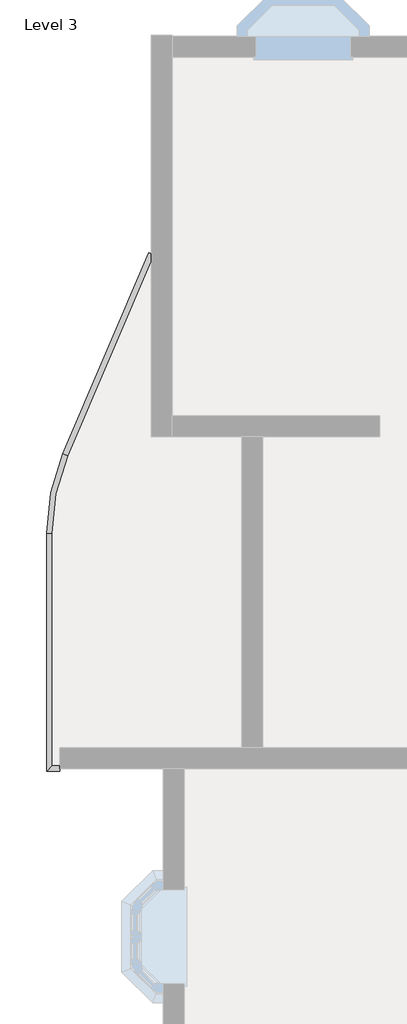
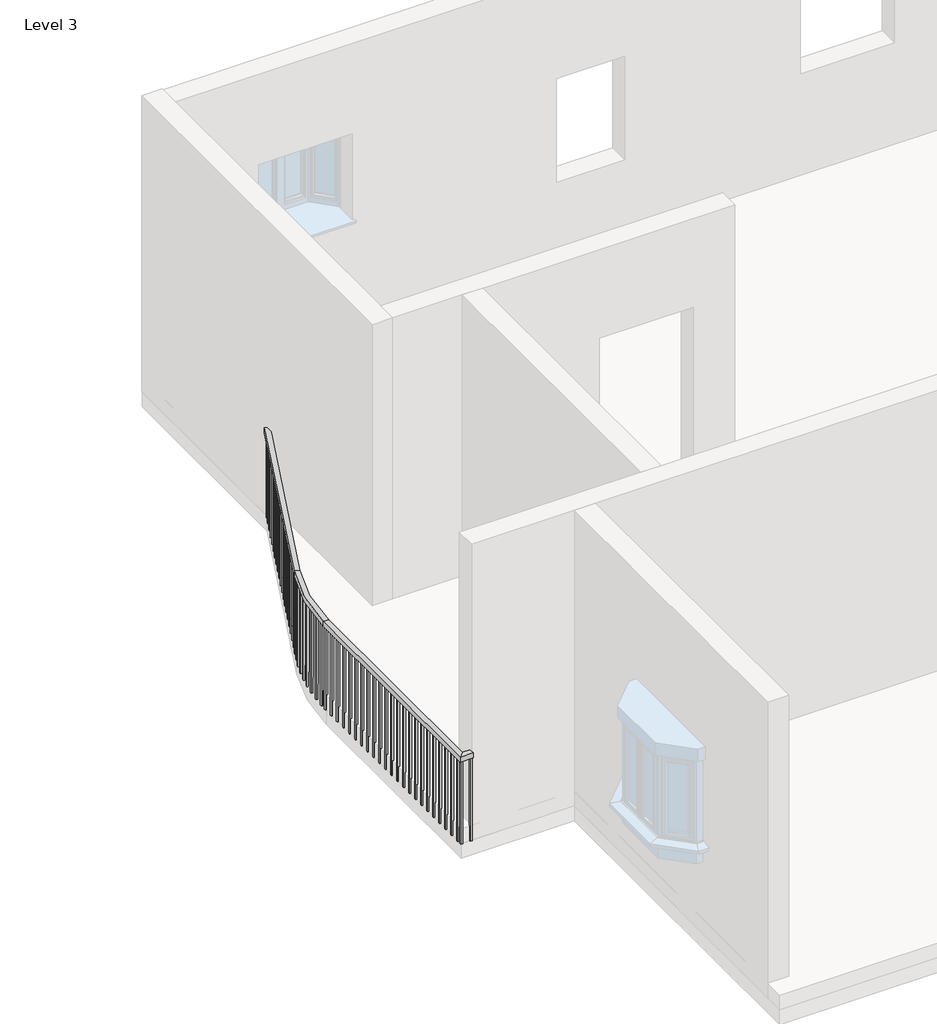
# One storey, part 7 of 14: 1 railing.
"""IFC4 building model written with IfcOpenShell, lengths in millimetres."""

from ifc_helpers import new_model, si_unit, frame, origin, place, context, project, spatial, polyline, circle_curve, outline, extrude, element, save
from ifc_brep_helpers import plane_surface, cylinder_surface, revolved_surface, advanced_brep

model = new_model("IFC4")

# Units and contexts
model_context = context("Model", 3, world=origin())
ifc_project = project(units=[si_unit("LENGTHUNIT", "METRE", prefix="MILLI")], contexts=[model_context])

# Site, building, storey
site = spatial("IfcSite", under=ifc_project)
building = spatial("IfcBuilding", under=site)
storey = spatial("IfcBuildingStorey", under=building, Name="Level 3", Elevation=6096.0)

# Railing
placement = place(None, origin())
element("IfcRailing", 1, ObjectType="Handrail - Rectangular", at=placement, inside=storey, context=model_context, shape_type="SolidModel", body=[
    advanced_brep(
    [(-12381.4379579, -2441.2590879, 7010.4), (-12381.4379579, -2441.2590879, 6959.6), (-12428.1364721, -2421.2618688, 6959.6), (-12428.1364721, -2421.2618688, 7010.4), (-13216.1814979, -4390.5942894, 7010.4), (-13216.1814979, -4390.5942894, 6959.6), (-13262.8800121, -4370.5970703, 6959.6), (-13262.8800121, -4370.5970703, 7010.4), (-13369.987215, -5140.4900045, 6959.6), (-13369.987215, -5140.4900045, 7010.4), (-13420.787215, -5140.4900045, 6959.6), (-13420.787215, -5140.4900045, 7010.4), (-13369.987215, -7396.5416506, 7010.4), (-13369.987215, -7396.5416506, 6959.6), (-13420.787215, -7447.3416506, 6959.6), (-13420.787215, -7447.3416506, 7010.4), (-13293.787215, -7396.5416506, 7010.4), (-13293.787215, -7447.3416506, 7010.4), (-13293.787215, -7447.3416506, 6959.6), (-13293.787215, -7396.5416506, 6959.6)],
    [
        (0, 1),
        (1, 2),
        (2, 3),
        (3, 0),
        (0, 4),
        (4, 5),
        (5, 1),
        (5, 6),
        (6, 2),
        (6, 7),
        (7, 3),
        (7, 4),
        (8, 5, circle_curve(frame((-11464.987215, -5140.4900045, 6959.6), z_axis=(0.0, 0.0, -1.0), x_axis=(-0.9192620907623801, 0.39364604467361003, 0.0)), 1905.0)),
        (4, 9, circle_curve(frame((-11464.987215, -5140.4900045, 7010.4), z_axis=(0.0, 0.0, 1.0), x_axis=(-0.9192620907623801, 0.39364604467361003, 0.0)), 1905.0)),
        (9, 8),
        (10, 6, circle_curve(frame((-11464.987215, -5140.4900045, 6959.6), z_axis=(0.0, 0.0, -1.0), x_axis=(-0.9192620907623801, 0.39364604467361003, 0.0)), 1955.8)),
        (8, 10),
        (11, 7, circle_curve(frame((-11464.987215, -5140.4900045, 7010.4), z_axis=(0.0, 0.0, -1.0), x_axis=(-0.9192620907623801, 0.39364604467361003, 0.0)), 1955.8)),
        (10, 11),
        (11, 9),
        (9, 12),
        (12, 13),
        (13, 8),
        (13, 14),
        (14, 10),
        (14, 15),
        (15, 11),
        (15, 12),
        (16, 17),
        (17, 18),
        (18, 19),
        (19, 16),
        (12, 16),
        (19, 13),
        (18, 14),
        (17, 15),
    ],
    [
        plane_surface(frame((-12404.787215, -2431.2604783, 7010.4), z_axis=(0.39364604467361003, 0.9192620907623801, 0.0), x_axis=(0.9192620907623801, -0.39364604467361003, 0.0))),
        plane_surface(frame((-12381.4379579, -2441.2590879, 7010.4), z_axis=(0.91926209076238, -0.39364604467361014, 0.0), x_axis=(-0.39364604467361014, -0.91926209076238, 0.0))),
        plane_surface(frame((-12381.4379579, -2441.2590879, 6959.6), z_axis=(0.0, 0.0, -1.0), x_axis=(-0.39364604467361014, -0.91926209076238, 0.0))),
        plane_surface(frame((-12428.1364721, -2421.2618688, 6959.6), z_axis=(-0.91926209076238, 0.39364604467361014, 0.0), x_axis=(-0.39364604467361014, -0.91926209076238, 0.0))),
        plane_surface(frame((-12428.1364721, -2421.2618688, 7010.4), z_axis=(0.0, 0.0, 1.0), x_axis=(-0.39364604467361014, -0.91926209076238, 0.0))),
        revolved_surface(polyline([(-13216.181497902333, -4390.594289396773, 7010.4), (-13216.181497902333, -4390.594289396773, 6959.6)]), (-11464.987215, -5140.4900045, 7010.4), (0.0, 0.0, 1.0)),
        plane_surface(frame((-11464.987215, -5140.4900045, 6959.6), z_axis=(0.0, 0.0, -1.0000000000000002), x_axis=(-0.9192620907623801, 0.39364604467361003, 0.0))),
        cylinder_surface(frame((-11464.987215, -5140.4900045, 7010.4), z_axis=(0.0, 0.0, 1.0), x_axis=(-0.9192620907623801, 0.39364604467361003, 0.0)), 1955.8),
        plane_surface(frame((-11464.987215, -5140.4900045, 7010.4), z_axis=(0.0, 0.0, 1.0000000000000002), x_axis=(-0.9192620907623801, 0.39364604467361003, 0.0))),
        plane_surface(frame((-13369.987215, -5140.4900045, 7010.4), z_axis=(1.0, 0.0, 0.0), x_axis=(0.0, -1.0, 0.0))),
        plane_surface(frame((-13369.987215, -5140.4900045, 6959.6), z_axis=(0.0, 0.0, -1.0), x_axis=(0.0, -1.0, 0.0))),
        plane_surface(frame((-13420.787215, -5140.4900045, 6959.6), z_axis=(-1.0, 0.0, 0.0), x_axis=(0.0, -1.0, 0.0))),
        plane_surface(frame((-13420.787215, -5140.4900045, 7010.4), z_axis=(0.0, 0.0, 1.0), x_axis=(0.0, -1.0, 0.0))),
        plane_surface(frame((-13293.787215, -7421.9416506, 7010.4), z_axis=(1.0, 0.0, 0.0), x_axis=(0.0, 1.0, 0.0))),
        plane_surface(frame((-13369.987215, -7396.5416506, 7010.4), z_axis=(0.0, 1.0, 0.0), x_axis=(1.0, 0.0, 0.0))),
        plane_surface(frame((-13369.987215, -7396.5416506, 6959.6), z_axis=(0.0, 0.0, -1.0), x_axis=(1.0, 0.0, 0.0))),
        plane_surface(frame((-13420.787215, -7447.3416506, 6959.6), z_axis=(0.0, -1.0, 0.0), x_axis=(1.0, 0.0, 0.0))),
        plane_surface(frame((-13420.787215, -7447.3416506, 7010.4), z_axis=(0.0, 0.0, 1.0), x_axis=(1.0, 0.0, 0.0))),
    ],
    [
        (0, [[1, 2, 3, 4]]),
        (1, [[-1, 5, 6, 7]]),
        (2, [[-2, -7, 8, 9]]),
        (3, [[-3, -9, 10, 11]]),
        (4, [[-4, -11, 12, -5]]),
        (5, [[13, -6, 14, 15]]),
        (6, [[16, -8, -13, 17]]),
        (7, [[18, -10, -16, 19]]),
        (8, [[-14, -12, -18, 20]]),
        (9, [[-15, 21, 22, 23]]),
        (10, [[-17, -23, 24, 25]]),
        (11, [[-19, -25, 26, 27]]),
        (12, [[-20, -27, 28, -21]]),
        (13, [[29, 30, 31, 32]]),
        (14, [[-22, 33, -32, 34]]),
        (15, [[-24, -34, -31, 35]]),
        (16, [[-26, -35, -30, 36]]),
        (17, [[-28, -36, -29, -33]]),
    ],
),
    extrude(outline(polyline([(-13404.912215, -7366.1650045), (-13385.862215, -7366.1650045), (-13385.862215, -7385.2150045), (-13404.912215, -7385.2150045), (-13404.912215, -7366.1650045)])), frame((0.0, 0.0, 6096.0), z_axis=(0.0, 0.0, 1.0), x_axis=(1.0, 0.0, 0.0)), (0.0, 0.0, 1.0), 863.6),
    extrude(outline(polyline([(-13404.912215, -7264.5650045), (-13385.862215, -7264.5650045), (-13385.862215, -7283.6150045), (-13404.912215, -7283.6150045), (-13404.912215, -7264.5650045)])), frame((0.0, 0.0, 6096.0), z_axis=(0.0, 0.0, 1.0), x_axis=(1.0, 0.0, 0.0)), (0.0, 0.0, 1.0), 863.6),
    extrude(outline(polyline([(-13404.912215, -7162.9650045), (-13385.862215, -7162.9650045), (-13385.862215, -7182.0150045), (-13404.912215, -7182.0150045), (-13404.912215, -7162.9650045)])), frame((0.0, 0.0, 6096.0), z_axis=(0.0, 0.0, 1.0), x_axis=(1.0, 0.0, 0.0)), (0.0, 0.0, 1.0), 863.6),
    extrude(outline(polyline([(-13404.912215, -7061.3650045), (-13385.862215, -7061.3650045), (-13385.862215, -7080.4150045), (-13404.912215, -7080.4150045), (-13404.912215, -7061.3650045)])), frame((0.0, 0.0, 6096.0), z_axis=(0.0, 0.0, 1.0), x_axis=(1.0, 0.0, 0.0)), (0.0, 0.0, 1.0), 863.6),
    extrude(outline(polyline([(-13404.912215, -6959.7650045), (-13385.862215, -6959.7650045), (-13385.862215, -6978.8150045), (-13404.912215, -6978.8150045), (-13404.912215, -6959.7650045)])), frame((0.0, 0.0, 6096.0), z_axis=(0.0, 0.0, 1.0), x_axis=(1.0, 0.0, 0.0)), (0.0, 0.0, 1.0), 863.6),
    extrude(outline(polyline([(-13404.912215, -6858.1650045), (-13385.862215, -6858.1650045), (-13385.862215, -6877.2150045), (-13404.912215, -6877.2150045), (-13404.912215, -6858.1650045)])), frame((0.0, 0.0, 6096.0), z_axis=(0.0, 0.0, 1.0), x_axis=(1.0, 0.0, 0.0)), (0.0, 0.0, 1.0), 863.6),
    extrude(outline(polyline([(-13404.912215, -6756.5650045), (-13385.862215, -6756.5650045), (-13385.862215, -6775.6150045), (-13404.912215, -6775.6150045), (-13404.912215, -6756.5650045)])), frame((0.0, 0.0, 6096.0), z_axis=(0.0, 0.0, 1.0), x_axis=(1.0, 0.0, 0.0)), (0.0, 0.0, 1.0), 863.6),
    extrude(outline(polyline([(-13404.912215, -6654.9650045), (-13385.862215, -6654.9650045), (-13385.862215, -6674.0150045), (-13404.912215, -6674.0150045), (-13404.912215, -6654.9650045)])), frame((0.0, 0.0, 6096.0), z_axis=(0.0, 0.0, 1.0), x_axis=(1.0, 0.0, 0.0)), (0.0, 0.0, 1.0), 863.6),
    extrude(outline(polyline([(-13404.912215, -6553.3650045), (-13385.862215, -6553.3650045), (-13385.862215, -6572.4150045), (-13404.912215, -6572.4150045), (-13404.912215, -6553.3650045)])), frame((0.0, 0.0, 6096.0), z_axis=(0.0, 0.0, 1.0), x_axis=(1.0, 0.0, 0.0)), (0.0, 0.0, 1.0), 863.6),
    extrude(outline(polyline([(-13404.912215, -6451.7650045), (-13385.862215, -6451.7650045), (-13385.862215, -6470.8150045), (-13404.912215, -6470.8150045), (-13404.912215, -6451.7650045)])), frame((0.0, 0.0, 6096.0), z_axis=(0.0, 0.0, 1.0), x_axis=(1.0, 0.0, 0.0)), (0.0, 0.0, 1.0), 863.6),
    extrude(outline(polyline([(-13404.912215, -6350.1650045), (-13385.862215, -6350.1650045), (-13385.862215, -6369.2150045), (-13404.912215, -6369.2150045), (-13404.912215, -6350.1650045)])), frame((0.0, 0.0, 6096.0), z_axis=(0.0, 0.0, 1.0), x_axis=(1.0, 0.0, 0.0)), (0.0, 0.0, 1.0), 863.6),
    extrude(outline(polyline([(-13404.912215, -6248.5650045), (-13385.862215, -6248.5650045), (-13385.862215, -6267.6150045), (-13404.912215, -6267.6150045), (-13404.912215, -6248.5650045)])), frame((0.0, 0.0, 6096.0), z_axis=(0.0, 0.0, 1.0), x_axis=(1.0, 0.0, 0.0)), (0.0, 0.0, 1.0), 863.6),
    extrude(outline(polyline([(-13404.912215, -6146.9650045), (-13385.862215, -6146.9650045), (-13385.862215, -6166.0150045), (-13404.912215, -6166.0150045), (-13404.912215, -6146.9650045)])), frame((0.0, 0.0, 6096.0), z_axis=(0.0, 0.0, 1.0), x_axis=(1.0, 0.0, 0.0)), (0.0, 0.0, 1.0), 863.6),
    extrude(outline(polyline([(-13404.912215, -6045.3650045), (-13385.862215, -6045.3650045), (-13385.862215, -6064.4150045), (-13404.912215, -6064.4150045), (-13404.912215, -6045.3650045)])), frame((0.0, 0.0, 6096.0), z_axis=(0.0, 0.0, 1.0), x_axis=(1.0, 0.0, 0.0)), (0.0, 0.0, 1.0), 863.6),
    extrude(outline(polyline([(-13404.912215, -5943.7650045), (-13385.862215, -5943.7650045), (-13385.862215, -5962.8150045), (-13404.912215, -5962.8150045), (-13404.912215, -5943.7650045)])), frame((0.0, 0.0, 6096.0), z_axis=(0.0, 0.0, 1.0), x_axis=(1.0, 0.0, 0.0)), (0.0, 0.0, 1.0), 863.6),
    extrude(outline(polyline([(-13404.912215, -5842.1650045), (-13385.862215, -5842.1650045), (-13385.862215, -5861.2150045), (-13404.912215, -5861.2150045), (-13404.912215, -5842.1650045)])), frame((0.0, 0.0, 6096.0), z_axis=(0.0, 0.0, 1.0), x_axis=(1.0, 0.0, 0.0)), (0.0, 0.0, 1.0), 863.6),
    extrude(outline(polyline([(-13404.912215, -5740.5650045), (-13385.862215, -5740.5650045), (-13385.862215, -5759.6150045), (-13404.912215, -5759.6150045), (-13404.912215, -5740.5650045)])), frame((0.0, 0.0, 6096.0), z_axis=(0.0, 0.0, 1.0), x_axis=(1.0, 0.0, 0.0)), (0.0, 0.0, 1.0), 863.6),
    extrude(outline(polyline([(-13404.912215, -5638.9650045), (-13385.862215, -5638.9650045), (-13385.862215, -5658.0150045), (-13404.912215, -5658.0150045), (-13404.912215, -5638.9650045)])), frame((0.0, 0.0, 6096.0), z_axis=(0.0, 0.0, 1.0), x_axis=(1.0, 0.0, 0.0)), (0.0, 0.0, 1.0), 863.6),
    extrude(outline(polyline([(-13404.912215, -5537.3650045), (-13385.862215, -5537.3650045), (-13385.862215, -5556.4150045), (-13404.912215, -5556.4150045), (-13404.912215, -5537.3650045)])), frame((0.0, 0.0, 6096.0), z_axis=(0.0, 0.0, 1.0), x_axis=(1.0, 0.0, 0.0)), (0.0, 0.0, 1.0), 863.6),
    extrude(outline(polyline([(-13404.912215, -5435.7650045), (-13385.862215, -5435.7650045), (-13385.862215, -5454.8150045), (-13404.912215, -5454.8150045), (-13404.912215, -5435.7650045)])), frame((0.0, 0.0, 6096.0), z_axis=(0.0, 0.0, 1.0), x_axis=(1.0, 0.0, 0.0)), (0.0, 0.0, 1.0), 863.6),
    extrude(outline(polyline([(-13404.912215, -5334.1650045), (-13385.862215, -5334.1650045), (-13385.862215, -5353.2150045), (-13404.912215, -5353.2150045), (-13404.912215, -5334.1650045)])), frame((0.0, 0.0, 6096.0), z_axis=(0.0, 0.0, 1.0), x_axis=(1.0, 0.0, 0.0)), (0.0, 0.0, 1.0), 863.6),
    extrude(outline(polyline([(-13404.912215, -5232.5650045), (-13385.862215, -5232.5650045), (-13385.862215, -5251.6150045), (-13404.912215, -5251.6150045), (-13404.912215, -5232.5650045)])), frame((0.0, 0.0, 6096.0), z_axis=(0.0, 0.0, 1.0), x_axis=(1.0, 0.0, 0.0)), (0.0, 0.0, 1.0), 863.6),
    extrude(outline(polyline([(-13403.2986616, -5060.8127369), (-13384.2611239, -5061.5016911), (-13384.9500781, -5080.5392288), (-13403.9876158, -5079.8502746), (-13403.2986616, -5060.8127369)])), frame((0.0, 0.0, 6096.0), z_axis=(0.0, 0.0, 1.0), x_axis=(1.0, 0.0, 0.0)), (0.0, 0.0, 1.0), 863.6),
    extrude(outline(polyline([(-13396.4230348, -4958.9537683), (-13377.4481028, -4960.6432816), (-13379.1376161, -4979.6182136), (-13398.1125481, -4977.9287003), (-13396.4230348, -4958.9537683)])), frame((0.0, 0.0, 6096.0), z_axis=(0.0, 0.0, 1.0), x_axis=(1.0, 0.0, 0.0)), (0.0, 0.0, 1.0), 863.6),
    extrude(outline(polyline([(-13384.1984052, -4857.5975541), (-13365.3386289, -4860.2829475), (-13368.0240223, -4879.1427238), (-13386.8837986, -4876.4573304), (-13384.1984052, -4857.5975541)])), frame((0.0, 0.0, 6096.0), z_axis=(0.0, 0.0, 1.0), x_axis=(1.0, 0.0, 0.0)), (0.0, 0.0, 1.0), 863.6),
    extrude(outline(polyline([(-13366.6586282, -4757.0247946), (-13347.9662387, -4760.698631), (-13351.6400752, -4779.3910205), (-13370.3324647, -4775.7171841), (-13366.6586282, -4757.0247946)])), frame((0.0, 0.0, 6096.0), z_axis=(0.0, 0.0, 1.0), x_axis=(1.0, 0.0, 0.0)), (0.0, 0.0, 1.0), 863.6),
    extrude(outline(polyline([(-13343.8522793, -4657.5140204), (-13325.3790441, -4662.1661254), (-13330.0311492, -4680.6393606), (-13348.5043844, -4675.9872556), (-13343.8522793, -4657.5140204)])), frame((0.0, 0.0, 6096.0), z_axis=(0.0, 0.0, 1.0), x_axis=(1.0, 0.0, 0.0)), (0.0, 0.0, 1.0), 863.6),
    extrude(outline(polyline([(-13315.8425193, -4559.340821), (-13297.6395991, -4564.9583109), (-13303.257089, -4583.1612312), (-13321.4600093, -4577.5437413), (-13315.8425193, -4559.340821)])), frame((0.0, 0.0, 6096.0), z_axis=(0.0, 0.0, 1.0), x_axis=(1.0, 0.0, 0.0)), (0.0, 0.0, 1.0), 863.6),
    extrude(outline(polyline([(-13282.7069198, -4462.7770815), (-13264.8247264, -4469.344399), (-13271.3920438, -4487.2265924), (-13289.2742372, -4480.659275), (-13282.7069198, -4462.7770815)])), frame((0.0, 0.0, 6096.0), z_axis=(0.0, 0.0, 1.0), x_axis=(1.0, 0.0, 0.0)), (0.0, 0.0, 1.0), 863.6),
    extrude(outline(polyline([(-13209.6824706, -4286.6955968), (-13192.1705278, -4294.1945539), (-13199.6694849, -4311.7064967), (-13217.1814277, -4304.2075396), (-13209.6824706, -4286.6955968)])), frame((0.0, 0.0, 6096.0), z_axis=(0.0, 0.0, 1.0), x_axis=(1.0, 0.0, 0.0)), (0.0, 0.0, 1.0), 863.6),
    extrude(outline(polyline([(-13169.6880325, -4193.2985683), (-13152.1760896, -4200.7975255), (-13159.6750468, -4218.3094683), (-13177.1869896, -4210.8105112), (-13169.6880325, -4193.2985683)])), frame((0.0, 0.0, 6096.0), z_axis=(0.0, 0.0, 1.0), x_axis=(1.0, 0.0, 0.0)), (0.0, 0.0, 1.0), 863.6),
    extrude(outline(polyline([(-13129.6935943, -4099.9015399), (-13112.1816515, -4107.4004971), (-13119.6806086, -4124.9124399), (-13137.1925515, -4117.4134827), (-13129.6935943, -4099.9015399)])), frame((0.0, 0.0, 6096.0), z_axis=(0.0, 0.0, 1.0), x_axis=(1.0, 0.0, 0.0)), (0.0, 0.0, 1.0), 863.6),
    extrude(outline(polyline([(-13089.6991562, -4006.5045115), (-13072.1872133, -4014.0034686), (-13079.6861705, -4031.5154115), (-13097.1981133, -4024.0164543), (-13089.6991562, -4006.5045115)])), frame((0.0, 0.0, 6096.0), z_axis=(0.0, 0.0, 1.0), x_axis=(1.0, 0.0, 0.0)), (0.0, 0.0, 1.0), 863.6),
    extrude(outline(polyline([(-13049.704718, -3913.1074831), (-13032.1927752, -3920.6064402), (-13039.6917324, -3938.1183831), (-13057.2036752, -3930.6194259), (-13049.704718, -3913.1074831)])), frame((0.0, 0.0, 6096.0), z_axis=(0.0, 0.0, 1.0), x_axis=(1.0, 0.0, 0.0)), (0.0, 0.0, 1.0), 863.6),
    extrude(outline(polyline([(-13009.7102799, -3819.7104546), (-12992.1983371, -3827.2094118), (-12999.6972942, -3844.7213546), (-13017.209237, -3837.2223975), (-13009.7102799, -3819.7104546)])), frame((0.0, 0.0, 6096.0), z_axis=(0.0, 0.0, 1.0), x_axis=(1.0, 0.0, 0.0)), (0.0, 0.0, 1.0), 863.6),
    extrude(outline(polyline([(-12969.7158418, -3726.3134262), (-12952.2038989, -3733.8123834), (-12959.7028561, -3751.3243262), (-12977.2147989, -3743.8253691), (-12969.7158418, -3726.3134262)])), frame((0.0, 0.0, 6096.0), z_axis=(0.0, 0.0, 1.0), x_axis=(1.0, 0.0, 0.0)), (0.0, 0.0, 1.0), 863.6),
    extrude(outline(polyline([(-12929.7214036, -3632.9163978), (-12912.2094608, -3640.415355), (-12919.7084179, -3657.9272978), (-12937.2203608, -3650.4283406), (-12929.7214036, -3632.9163978)])), frame((0.0, 0.0, 6096.0), z_axis=(0.0, 0.0, 1.0), x_axis=(1.0, 0.0, 0.0)), (0.0, 0.0, 1.0), 863.6),
    extrude(outline(polyline([(-12889.7269655, -3539.5193694), (-12872.2150227, -3547.0183265), (-12879.7139798, -3564.5302694), (-12897.2259226, -3557.0313122), (-12889.7269655, -3539.5193694)])), frame((0.0, 0.0, 6096.0), z_axis=(0.0, 0.0, 1.0), x_axis=(1.0, 0.0, 0.0)), (0.0, 0.0, 1.0), 863.6),
    extrude(outline(polyline([(-12849.7325273, -3446.122341), (-12832.2205845, -3453.6212981), (-12839.7195417, -3471.1332409), (-12857.2314845, -3463.6342838), (-12849.7325273, -3446.122341)])), frame((0.0, 0.0, 6096.0), z_axis=(0.0, 0.0, 1.0), x_axis=(1.0, 0.0, 0.0)), (0.0, 0.0, 1.0), 863.6),
    extrude(outline(polyline([(-12809.7380892, -3352.7253125), (-12792.2261464, -3360.2242697), (-12799.7251035, -3377.7362125), (-12817.2370464, -3370.2372554), (-12809.7380892, -3352.7253125)])), frame((0.0, 0.0, 6096.0), z_axis=(0.0, 0.0, 1.0), x_axis=(1.0, 0.0, 0.0)), (0.0, 0.0, 1.0), 863.6),
    extrude(outline(polyline([(-12769.7436511, -3259.3282841), (-12752.2317082, -3266.8272413), (-12759.7306654, -3284.3391841), (-12777.2426082, -3276.8402269), (-12769.7436511, -3259.3282841)])), frame((0.0, 0.0, 6096.0), z_axis=(0.0, 0.0, 1.0), x_axis=(1.0, 0.0, 0.0)), (0.0, 0.0, 1.0), 863.6),
    extrude(outline(polyline([(-12729.7492129, -3165.9312557), (-12712.2372701, -3173.4302129), (-12719.7362272, -3190.9421557), (-12737.2481701, -3183.4431985), (-12729.7492129, -3165.9312557)])), frame((0.0, 0.0, 6096.0), z_axis=(0.0, 0.0, 1.0), x_axis=(1.0, 0.0, 0.0)), (0.0, 0.0, 1.0), 863.6),
    extrude(outline(polyline([(-12689.7547748, -3072.5342273), (-12672.242832, -3080.0331844), (-12679.7417891, -3097.5451273), (-12697.2537319, -3090.0461701), (-12689.7547748, -3072.5342273)])), frame((0.0, 0.0, 6096.0), z_axis=(0.0, 0.0, 1.0), x_axis=(1.0, 0.0, 0.0)), (0.0, 0.0, 1.0), 863.6),
    extrude(outline(polyline([(-12649.7603366, -2979.1371989), (-12632.2483938, -2986.636156), (-12639.747351, -3004.1480988), (-12657.2592938, -2996.6491417), (-12649.7603366, -2979.1371989)])), frame((0.0, 0.0, 6096.0), z_axis=(0.0, 0.0, 1.0), x_axis=(1.0, 0.0, 0.0)), (0.0, 0.0, 1.0), 863.6),
    extrude(outline(polyline([(-12609.7658985, -2885.7401704), (-12592.2539557, -2893.2391276), (-12599.7529128, -2910.7510704), (-12617.2648557, -2903.2521133), (-12609.7658985, -2885.7401704)])), frame((0.0, 0.0, 6096.0), z_axis=(0.0, 0.0, 1.0), x_axis=(1.0, 0.0, 0.0)), (0.0, 0.0, 1.0), 863.6),
    extrude(outline(polyline([(-12569.7714604, -2792.343142), (-12552.2595175, -2799.8420992), (-12559.7584747, -2817.354042), (-12577.2704175, -2809.8550848), (-12569.7714604, -2792.343142)])), frame((0.0, 0.0, 6096.0), z_axis=(0.0, 0.0, 1.0), x_axis=(1.0, 0.0, 0.0)), (0.0, 0.0, 1.0), 863.6),
    extrude(outline(polyline([(-12529.7770222, -2698.9461136), (-12512.2650794, -2706.4450707), (-12519.7640366, -2723.9570136), (-12537.2759794, -2716.4580564), (-12529.7770222, -2698.9461136)])), frame((0.0, 0.0, 6096.0), z_axis=(0.0, 0.0, 1.0), x_axis=(1.0, 0.0, 0.0)), (0.0, 0.0, 1.0), 863.6),
    extrude(outline(polyline([(-12489.7825841, -2605.5490852), (-12472.2706413, -2613.0480423), (-12479.7695984, -2630.5599852), (-12497.2815412, -2623.061028), (-12489.7825841, -2605.5490852)])), frame((0.0, 0.0, 6096.0), z_axis=(0.0, 0.0, 1.0), x_axis=(1.0, 0.0, 0.0)), (0.0, 0.0, 1.0), 863.6),
    extrude(outline(polyline([(-12449.788146, -2512.1520567), (-12432.2762031, -2519.6510139), (-12439.7751603, -2537.1629567), (-12457.2871031, -2529.6639996), (-12449.788146, -2512.1520567)])), frame((0.0, 0.0, 6096.0), z_axis=(0.0, 0.0, 1.0), x_axis=(1.0, 0.0, 0.0)), (0.0, 0.0, 1.0), 863.6),
    extrude(outline(polyline([(-13404.912215, -7412.4166506), (-13385.862215, -7412.4166506), (-13385.862215, -7431.4666506), (-13404.912215, -7431.4666506), (-13404.912215, -7412.4166506)])), frame((0.0, 0.0, 6096.0), z_axis=(0.0, 0.0, 1.0), x_axis=(1.0, 0.0, 0.0)), (0.0, 0.0, 1.0), 863.6),
    extrude(outline(polyline([(-13404.912215, -5130.9650045), (-13385.862215, -5130.9650045), (-13385.862215, -5150.0150045), (-13404.912215, -5150.0150045), (-13404.912215, -5130.9650045)])), frame((0.0, 0.0, 6096.0), z_axis=(0.0, 0.0, 1.0), x_axis=(1.0, 0.0, 0.0)), (0.0, 0.0, 1.0), 863.6),
    extrude(outline(polyline([(-13244.5372478, -4368.0902299), (-13227.025305, -4375.589187), (-13234.5242621, -4393.1011299), (-13252.036205, -4385.6021727), (-13244.5372478, -4368.0902299)])), frame((0.0, 0.0, 6096.0), z_axis=(0.0, 0.0, 1.0), x_axis=(1.0, 0.0, 0.0)), (0.0, 0.0, 1.0), 863.6),
    extrude(outline(polyline([(-13312.837215, -7431.4666506), (-13312.837215, -7412.4166506), (-13293.787215, -7412.4166506), (-13293.787215, -7431.4666506), (-13312.837215, -7431.4666506)])), frame((0.0, 0.0, 6096.0), z_axis=(0.0, 0.0, 1.0), x_axis=(1.0, 0.0, 0.0)), (0.0, 0.0, 1.0), 863.6),
    extrude(outline(polyline([(-12413.5431864, -2427.5109997), (-12396.0312436, -2435.0099569), (-12403.5302007, -2452.5218997), (-12421.0421435, -2445.0229426), (-12413.5431864, -2427.5109997)])), frame((0.0, 0.0, 6096.0), z_axis=(0.0, 0.0, 1.0), x_axis=(1.0, 0.0, 0.0)), (0.0, 0.0, 1.0), 863.6),
])

save(model, "model.ifc")

# Revit data of these elements
# Type "Handrail - Rectangular"
#   Assembly Code = "C2010400"
#   built-in parameter 1008612 = 0.0416667 (stored number, unit not read)
#   built-in parameter 1008611 = 0.0416667 (stored number, unit not read)
#   built-in parameter 1008609 = 0.333333 (stored number, unit not read)
#   built-in parameter 1008604 = 0.166667 (stored number, unit not read)
#   built-in parameter 1008603 = 0.166667 (stored number, unit not read)
#   Railing Height = 3' - 0"
#   built-in parameter 1008630 = 2
#   built-in parameter 1008610 = 2
#   built-in parameter 1008618 = Baluster - Square : 3/4"
# Element 1 (IfcRailing, "Handrail - Rectangular")
#   Phase Created = New Construction
